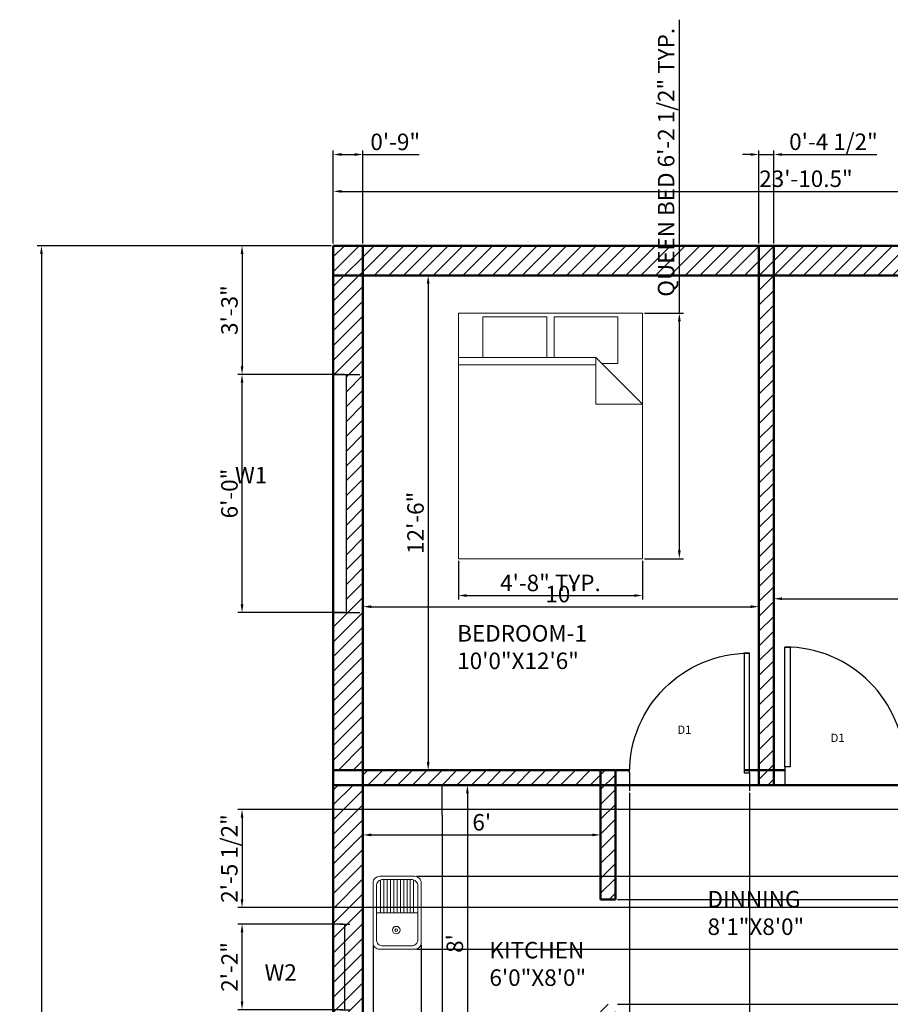
# Model space of a CAD drawing. Units: millimetres. Extents: x 2600 to 3013, y 1440 to 2066.
# Tile 3 of 4: x 2600 to 2864, y 1768 to 2066. Entities that reach past the tile are written whole.
import ezdxf

# ---------------------------------------------------------------- set-up
doc = ezdxf.new("R2010")
doc.units = ezdxf.units.MM
for name, color, linetype, lineweight in [('A-AREA-IDEN', 130, 'Continuous', 25), ('A-FLOR-CASE', 8, 'Continuous', 25), ('A-FLOR-FIXT', 160, 'Continuous', 18), ('A-WALL-PATT', 90, 'Continuous', 13), ('dimensions', 50, 'Continuous', 18), ('doors', 200, 'Continuous', 25), ('furniture', 160, 'Continuous', 18), ('text', 130, 'Continuous', 18), ('walls', 90, 'Continuous', 50), ('windows', 30, 'Continuous', 25)]:
    doc.layers.add(name, color=color, linetype=linetype, lineweight=lineweight)
doc.styles.get("Standard").update_dxf_attribs({"font": 'arial.ttf'})
doc.dimstyles.new('ISO-25', dxfattribs={"dimtxt": 5, "dimasz": 2.5, "dimexe": 1.25, "dimexo": 0.625, "dimtad": 1, "dimdec": 1, "dimlunit": 3, "dimtxsty": 'Standard', "dimcen": 2.5, "dimadec": 0, "dimazin": 0, "dimtfac": 1, "dimtdec": 1, "dimtmove": 0, "dimatfit": 3, "dimfxl": 1, "dimarcsym": 0})

# ---------------------------------------------------------------- blocks, each defined once
blk = doc.blocks.new('*U2')
for p, q in [((0, 0), (0, -6)), ((40, 0), (40, -6))]:
    blk.add_line(p, q)
blk.add_lwpolyline([(0, 0), (0, 40), (1.75, 40), (1.75, 0)], close=True)
blk.add_arc((0, 0), 40, 0, 90)
blk = doc.blocks.new('*U4')
for p, q in [((0, 4), (0, 0)), ((0, 2), (36, 2)), ((36, 4), (36, 0))]:
    blk.add_line(p, q)
blk = doc.blocks.new('*U6')
for p, q in [((0, 4), (0, 0)), ((36, 4), (36, 0)), ((0, 2), (36, 2))]:
    blk.add_line(p, q)
blk = doc.blocks.new('Bed - Queen')
for p, q in [((0, -80.00003), (0, 0)), ((0, 0), (59.99999, 0)), ((59.99999, 0), (59.99999, -80.00003)), ((7.99999, -1.2), (28.79998, -1.2)), ((7.99999, -14.4), (7.99999, -1.2)), ((28.79998, -1.2), (28.79998, -14.4)), ((31.19999, -1.2), (51.99999, -1.2)), ((31.19999, -14.4), (31.19999, -1.2)), ((51.99999, -1.2), (51.99999, -16.4)), ((0, -14.4), (44.8, -14.4)), ((59.99999, -29.6), (44.8, -14.4)), ((44.8, -14.4), (44.8, -29.6)), ((44.8, -16.8), (0, -16.8)), ((51.99999, -16.4), (46.79936, -16.4)), ((44.8, -29.6), (59.99999, -29.6)), ((59.99999, -80.00003), (0, -80.00003))]:
    blk.add_line(p, q)
blk = doc.blocks.new('*D10')
at = {"layer": 'Defpoints', "color": 0, "transparency": 16777216}
for p in [(2703.76, 1895.81), (2823.76, 1895.81), (2823.76, 1888.27)]:
    blk.add_point(p, dxfattribs=at)
at = {"layer": 'dimensions', "color": 0, "lineweight": -2, "transparency": 16777216}
for p, q in [((2703.76, 1895.19), (2703.76, 1887.02)), ((2823.76, 1895.19), (2823.76, 1887.02)), ((2706.26, 1888.27), (2821.26, 1888.27))]:
    blk.add_line(p, q, dxfattribs=at)
at = {"layer": 'dimensions', "color": 0, "transparency": 16777216}
for points in [[(2706.26, 1888.69), (2706.26, 1887.86), (2703.76, 1888.27)], [(2821.26, 1888.69), (2821.26, 1887.86), (2823.76, 1888.27)]]:
    blk.add_solid(points, dxfattribs=at)
at = {"layer": 'dimensions', "color": 0, "transparency": 16777216, "insert": (2763.76, 1891.45), "char_height": 5, "attachment_point": 5}
blk.add_mtext("10'", dxfattribs=at)
blk = doc.blocks.new('*D11')
at = {"layer": 'Defpoints', "color": 0, "transparency": 16777216}
for p in [(2714.32, 1988.68), (2714.32, 1838.68), (2723.51, 1838.68)]:
    blk.add_point(p, dxfattribs=at)
at = {"layer": 'dimensions', "color": 0, "lineweight": -2, "transparency": 16777216}
for p, q in [((2714.95, 1988.68), (2724.76, 1988.68)), ((2723.51, 1986.18), (2723.51, 1841.18)), ((2714.95, 1838.68), (2724.76, 1838.68))]:
    blk.add_line(p, q, dxfattribs=at)
at = {"layer": 'dimensions', "color": 0, "transparency": 16777216}
for points in [[(2723.1, 1986.18), (2723.93, 1986.18), (2723.51, 1988.68)], [(2723.1, 1841.18), (2723.93, 1841.18), (2723.51, 1838.68)]]:
    blk.add_solid(points, dxfattribs=at)
at = {"layer": 'dimensions', "color": 0, "transparency": 16777216, "insert": (2720.34, 1913.68), "char_height": 5, "attachment_point": 5, "rotation": 90}
blk.add_mtext('12\'-6"', dxfattribs=at)
blk = doc.blocks.new('*D12')
at = {"layer": 'Defpoints', "color": 0, "transparency": 16777216}
for p in [(2828.26, 1889.98), (2972.26, 1890.68), (2972.26, 1890.68)]:
    blk.add_point(p, dxfattribs=at)
at = {"layer": 'dimensions', "color": 0, "lineweight": -2, "transparency": 16777216}
for p, q in [((2828.26, 1890.6), (2828.26, 1891.93)), ((2830.76, 1890.68), (2969.76, 1890.68)), ((2972.26, 1891.3), (2972.26, 1891.93))]:
    blk.add_line(p, q, dxfattribs=at)
at = {"layer": 'dimensions', "color": 0, "transparency": 16777216}
for points in [[(2830.76, 1891.1), (2830.76, 1890.26), (2828.26, 1890.68)], [(2969.76, 1891.1), (2969.76, 1890.26), (2972.26, 1890.68)]]:
    blk.add_solid(points, dxfattribs=at)
at = {"layer": 'dimensions', "color": 0, "transparency": 16777216, "insert": (2900.26, 1893.81), "char_height": 5, "attachment_point": 5}
blk.add_mtext("12'", dxfattribs=at)
blk = doc.blocks.new('*D14')
at = {"layer": 'Defpoints', "color": 0, "transparency": 16777216}
for p in [(2735.41, 1834.18), (2735.41, 1738.18), (2735.41, 1738.18)]:
    blk.add_point(p, dxfattribs=at)
at = {"layer": 'dimensions', "color": 0, "lineweight": -2, "transparency": 16777216}
for p, q in [((2736.04, 1834.18), (2736.66, 1834.18)), ((2735.41, 1831.68), (2735.41, 1740.68)), ((2736.04, 1738.18), (2736.66, 1738.18))]:
    blk.add_line(p, q, dxfattribs=at)
at = {"layer": 'dimensions', "color": 0, "transparency": 16777216}
for points in [[(2735, 1831.68), (2735.83, 1831.68), (2735.41, 1834.18)], [(2735, 1740.68), (2735.83, 1740.68), (2735.41, 1738.18)]]:
    blk.add_solid(points, dxfattribs=at)
at = {"layer": 'dimensions', "color": 0, "transparency": 16777216, "insert": (2732.24, 1786.18), "char_height": 5, "attachment_point": 5, "rotation": 90}
blk.add_mtext("8'", dxfattribs=at)
blk = doc.blocks.new('*D15')
at = {"layer": 'Defpoints', "color": 0, "transparency": 16777216}
for p in [(2703.76, 1826.2), (2775.76, 1826.2), (2775.76, 1819.09)]:
    blk.add_point(p, dxfattribs=at)
at = {"layer": 'dimensions', "color": 0, "lineweight": -2, "transparency": 16777216}
for p, q in [((2703.76, 1825.58), (2703.76, 1817.84)), ((2775.76, 1825.58), (2775.76, 1817.84)), ((2706.26, 1819.09), (2773.26, 1819.09))]:
    blk.add_line(p, q, dxfattribs=at)
at = {"layer": 'dimensions', "color": 0, "transparency": 16777216}
for points in [[(2706.26, 1819.51), (2706.26, 1818.67), (2703.76, 1819.09)], [(2773.26, 1819.51), (2773.26, 1818.67), (2775.76, 1819.09)]]:
    blk.add_solid(points, dxfattribs=at)
at = {"layer": 'dimensions', "color": 0, "transparency": 16777216, "insert": (2739.76, 1822.27), "char_height": 5, "attachment_point": 5}
blk.add_mtext("6'", dxfattribs=at)
blk = doc.blocks.new('*D27')
at = {"layer": 'Defpoints', "color": 0, "transparency": 16777216}
for p in [(2981.26, 2014.15), (2694.76, 1997.68), (2981.26, 1997.68)]:
    blk.add_point(p, dxfattribs=at)
at = {"layer": 'dimensions', "color": 0, "lineweight": -2, "transparency": 16777216}
for p, q in [((2694.76, 1998.3), (2694.76, 2015.4)), ((2981.26, 1998.3), (2981.26, 2015.4)), ((2697.26, 2014.15), (2978.76, 2014.15))]:
    blk.add_line(p, q, dxfattribs=at)
at = {"layer": 'dimensions', "color": 0, "transparency": 16777216}
for points in [[(2697.26, 2014.57), (2697.26, 2013.74), (2694.76, 2014.15)], [(2978.76, 2014.57), (2978.76, 2013.74), (2981.26, 2014.15)]]:
    blk.add_solid(points, dxfattribs=at)
at = {"layer": 'dimensions', "color": 0, "transparency": 16777216, "insert": (2838.01, 2017.33), "char_height": 5, "attachment_point": 5}
blk.add_mtext('23\'-10.5"', dxfattribs=at)
blk = doc.blocks.new('*D28')
at = {"layer": 'Defpoints', "color": 0, "transparency": 16777216}
for p in [(2694.76, 1997.68), (2606.3, 1506.18), (2694.76, 1506.18)]:
    blk.add_point(p, dxfattribs=at)
at = {"layer": 'dimensions', "color": 0, "lineweight": -2, "transparency": 16777216}
for p, q in [((2694.13, 1997.68), (2605.05, 1997.68)), ((2606.3, 1995.18), (2606.3, 1508.68)), ((2694.13, 1506.18), (2605.05, 1506.18))]:
    blk.add_line(p, q, dxfattribs=at)
at = {"layer": 'dimensions', "color": 0, "transparency": 16777216}
for points in [[(2605.88, 1995.18), (2606.72, 1995.18), (2606.3, 1997.68)], [(2605.88, 1508.68), (2606.72, 1508.68), (2606.3, 1506.18)]]:
    blk.add_solid(points, dxfattribs=at)
at = {"layer": 'dimensions', "color": 0, "transparency": 16777216, "insert": (2603.12, 1751.93), "char_height": 5, "attachment_point": 5, "rotation": 90}
blk.add_mtext('40\'-11.5"', dxfattribs=at)
blk = doc.blocks.new('*D29')
at = {"layer": 'Defpoints', "color": 0, "transparency": 16777216}
for p in [(2788.48, 1977.23), (2799.64, 1977.23), (2788.48, 1902.81)]:
    blk.add_point(p, dxfattribs=at)
at = {"layer": 'dimensions', "color": 0, "lineweight": -2, "transparency": 16777216}
for p, q in [((2799.64, 1977.23), (2799.64, 2066.19)), ((2789.1, 1977.23), (2800.89, 1977.23)), ((2799.64, 1905.31), (2799.64, 1974.73)), ((2789.1, 1902.81), (2800.89, 1902.81))]:
    blk.add_line(p, q, dxfattribs=at)
at = {"layer": 'dimensions', "color": 0, "transparency": 16777216}
for points in [[(2799.22, 1974.73), (2800.06, 1974.73), (2799.64, 1977.23)], [(2799.22, 1905.31), (2800.06, 1905.31), (2799.64, 1902.81)]]:
    blk.add_solid(points, dxfattribs=at)
at = {"layer": 'dimensions', "color": 0, "transparency": 16777216, "insert": (2796.28, 2022.96), "char_height": 5, "attachment_point": 5, "rotation": 90}
blk.add_mtext('QUEEN BED 6\'-2 1/2" TYP.', dxfattribs=at)
blk = doc.blocks.new('*D30')
at = {"layer": 'Defpoints', "color": 0, "transparency": 16777216}
for p in [(2732.66, 1902.81), (2788.48, 1902.81), (2788.48, 1891.65)]:
    blk.add_point(p, dxfattribs=at)
at = {"layer": 'dimensions', "color": 0, "lineweight": -2, "transparency": 16777216}
for p, q in [((2732.66, 1902.19), (2732.66, 1890.4)), ((2788.48, 1902.19), (2788.48, 1890.4)), ((2735.16, 1891.65), (2785.98, 1891.65))]:
    blk.add_line(p, q, dxfattribs=at)
at = {"layer": 'dimensions', "color": 0, "transparency": 16777216}
for points in [[(2735.16, 1892.07), (2735.16, 1891.23), (2732.66, 1891.65)], [(2785.98, 1892.07), (2785.98, 1891.23), (2788.48, 1891.65)]]:
    blk.add_solid(points, dxfattribs=at)
at = {"layer": 'dimensions', "color": 0, "transparency": 16777216, "insert": (2760.57, 1894.83), "char_height": 5, "attachment_point": 5}
blk.add_mtext('4\'-8" TYP.', dxfattribs=at)
blk = doc.blocks.new('*D38')
at = {"layer": 'Defpoints', "color": 0, "transparency": 16777216}
for p in [(2703.76, 2025.33), (2694.76, 1997.68), (2703.76, 1997.68)]:
    blk.add_point(p, dxfattribs=at)
at = {"layer": 'dimensions', "color": 0, "lineweight": -2, "transparency": 16777216}
for p, q in [((2694.76, 1998.3), (2694.76, 2026.58)), ((2703.76, 1998.3), (2703.76, 2026.58)), ((2697.26, 2025.33), (2701.26, 2025.33)), ((2703.76, 2025.33), (2720.8, 2025.33))]:
    blk.add_line(p, q, dxfattribs=at)
at = {"layer": 'dimensions', "color": 0, "transparency": 16777216}
for points in [[(2697.26, 2025.75), (2697.26, 2024.91), (2694.76, 2025.33)], [(2701.26, 2025.75), (2701.26, 2024.91), (2703.76, 2025.33)]]:
    blk.add_solid(points, dxfattribs=at)
at = {"layer": 'dimensions', "color": 0, "transparency": 16777216, "insert": (2713.53, 2028.51), "char_height": 5, "attachment_point": 5}
blk.add_mtext('0\'-9"', dxfattribs=at)
blk = doc.blocks.new('*D39')
at = {"layer": 'Defpoints', "color": 0, "transparency": 16777216}
for p in [(2828.26, 2025.33), (2823.76, 1997.68), (2828.26, 1997.68)]:
    blk.add_point(p, dxfattribs=at)
at = {"layer": 'dimensions', "color": 0, "lineweight": -2, "transparency": 16777216}
for p, q in [((2823.76, 1998.3), (2823.76, 2026.58)), ((2828.26, 1998.3), (2828.26, 2026.58)), ((2821.26, 2025.33), (2818.76, 2025.33)), ((2823.76, 2025.33), (2828.26, 2025.33)), ((2830.76, 2025.33), (2859.45, 2025.33))]:
    blk.add_line(p, q, dxfattribs=at)
at = {"layer": 'dimensions', "color": 0, "transparency": 16777216}
for points in [[(2821.26, 2025.75), (2821.26, 2024.91), (2823.76, 2025.33)], [(2830.76, 2025.75), (2830.76, 2024.91), (2828.26, 2025.33)]]:
    blk.add_solid(points, dxfattribs=at)
at = {"layer": 'dimensions', "color": 0, "transparency": 16777216, "insert": (2846.35, 2028.54), "char_height": 5, "attachment_point": 5}
blk.add_mtext('0\'-4 1/2"', dxfattribs=at)
blk = doc.blocks.new('*D40')
at = {"layer": 'Defpoints', "color": 0, "transparency": 16777216}
for p in [(2667.11, 1958.65), (2698.77, 1958.65), (2698.77, 1886.48)]:
    blk.add_point(p, dxfattribs=at)
at = {"layer": 'dimensions', "color": 0, "lineweight": -2, "transparency": 16777216}
for p, q in [((2698.14, 1958.65), (2665.86, 1958.65)), ((2667.11, 1888.98), (2667.11, 1956.15)), ((2698.14, 1886.48), (2665.86, 1886.48))]:
    blk.add_line(p, q, dxfattribs=at)
at = {"layer": 'dimensions', "color": 0, "transparency": 16777216}
for points in [[(2666.69, 1956.15), (2667.52, 1956.15), (2667.11, 1958.65)], [(2666.69, 1888.98), (2667.52, 1888.98), (2667.11, 1886.48)]]:
    blk.add_solid(points, dxfattribs=at)
at = {"layer": 'dimensions', "color": 0, "transparency": 16777216, "insert": (2663.93, 1922.56), "char_height": 5, "attachment_point": 5, "rotation": 90}
blk.add_mtext('6\'-0"', dxfattribs=at)
blk = doc.blocks.new('*D41')
at = {"layer": 'Defpoints', "color": 0, "transparency": 16777216}
for p in [(2667.11, 1792.07), (2698.28, 1792.07), (2698.28, 1766.09)]:
    blk.add_point(p, dxfattribs=at)
at = {"layer": 'dimensions', "color": 0, "lineweight": -2, "transparency": 16777216}
for p, q in [((2697.66, 1792.07), (2665.86, 1792.07)), ((2667.11, 1768.59), (2667.11, 1789.57)), ((2697.66, 1766.09), (2665.86, 1766.09))]:
    blk.add_line(p, q, dxfattribs=at)
at = {"layer": 'dimensions', "color": 0, "transparency": 16777216}
for points in [[(2666.69, 1789.57), (2667.52, 1789.57), (2667.11, 1792.07)], [(2666.69, 1768.59), (2667.52, 1768.59), (2667.11, 1766.09)]]:
    blk.add_solid(points, dxfattribs=at)
at = {"layer": 'dimensions', "color": 0, "transparency": 16777216, "insert": (2663.97, 1779.08), "char_height": 5, "attachment_point": 5, "rotation": 90}
blk.add_mtext('2\'-2"', dxfattribs=at)
blk = doc.blocks.new('*D43')
at = {"layer": 'Defpoints', "color": 0, "transparency": 16777216}
for p in [(2784.55, 1832.44), (2820.86, 1832.44), (2820.86, 1444.53)]:
    blk.add_point(p, dxfattribs=at)
at = {"layer": 'dimensions', "color": 0, "lineweight": -2, "transparency": 16777216}
for p, q in [((2784.55, 1831.81), (2784.55, 1443.28)), ((2820.86, 1831.81), (2820.86, 1443.28)), ((2787.05, 1444.53), (2818.36, 1444.53))]:
    blk.add_line(p, q, dxfattribs=at)
at = {"layer": 'dimensions', "color": 0, "transparency": 16777216}
for points in [[(2787.05, 1444.94), (2787.05, 1444.11), (2784.55, 1444.53)], [(2818.36, 1444.94), (2818.36, 1444.11), (2820.86, 1444.53)]]:
    blk.add_solid(points, dxfattribs=at)
at = {"layer": 'dimensions', "color": 0, "transparency": 16777216, "insert": (2802.7, 1447.74), "char_height": 5, "attachment_point": 5}
blk.add_mtext('3\'-0 1/2"', dxfattribs=at)
blk = doc.blocks.new('*D44')
at = {"layer": 'Defpoints', "color": 0, "transparency": 16777216}
for p in [(2883.26, 1826.8), (2667.11, 1797.08), (2883.26, 1797.08)]:
    blk.add_point(p, dxfattribs=at)
at = {"layer": 'dimensions', "color": 0, "lineweight": -2, "transparency": 16777216}
for p, q in [((2882.63, 1826.8), (2665.86, 1826.8)), ((2667.11, 1824.3), (2667.11, 1799.58)), ((2882.63, 1797.08), (2665.86, 1797.08))]:
    blk.add_line(p, q, dxfattribs=at)
at = {"layer": 'dimensions', "color": 0, "transparency": 16777216}
for points in [[(2666.69, 1824.3), (2667.52, 1824.3), (2667.11, 1826.8)], [(2666.69, 1799.58), (2667.52, 1799.58), (2667.11, 1797.08)]]:
    blk.add_solid(points, dxfattribs=at)
at = {"layer": 'dimensions', "color": 0, "transparency": 16777216, "insert": (2663.9, 1811.94), "char_height": 5, "attachment_point": 5, "rotation": 90}
blk.add_mtext('2\'-5 1/2"', dxfattribs=at)
blk = doc.blocks.new('*D47')
at = {"layer": 'Defpoints', "color": 0, "transparency": 16777216}
for p in [(2780.26, 1799.5), (3008.91, 1799.5), (2780.26, 1767.75)]:
    blk.add_point(p, dxfattribs=at)
at = {"layer": 'dimensions', "color": 0, "lineweight": -2, "transparency": 16777216}
for p, q in [((2780.88, 1799.5), (3010.16, 1799.5)), ((3008.91, 1770.25), (3008.91, 1797)), ((2780.88, 1767.75), (3010.16, 1767.75))]:
    blk.add_line(p, q, dxfattribs=at)
at = {"layer": 'dimensions', "color": 0, "transparency": 16777216}
for points in [[(3008.49, 1797), (3009.32, 1797), (3008.91, 1799.5)], [(3008.49, 1770.25), (3009.32, 1770.25), (3008.91, 1767.75)]]:
    blk.add_solid(points, dxfattribs=at)
at = {"layer": 'dimensions', "color": 0, "transparency": 16777216, "insert": (3005.73, 1783.63), "char_height": 5, "attachment_point": 5, "rotation": 90}
blk.add_mtext('2\'-8"', dxfattribs=at)
blk = doc.blocks.new('*D48')
at = {"layer": 'Defpoints', "color": 0, "transparency": 16777216}
for p in [(2706.82, 1786.43), (2721.39, 1786.43), (2721.39, 1444.53)]:
    blk.add_point(p, dxfattribs=at)
at = {"layer": 'dimensions', "color": 0, "lineweight": -2, "transparency": 16777216}
for p, q in [((2706.82, 1785.8), (2706.82, 1443.28)), ((2721.39, 1785.8), (2721.39, 1443.28)), ((2709.32, 1444.53), (2718.89, 1444.53)), ((2721.39, 1444.53), (2749.61, 1444.53))]:
    blk.add_line(p, q, dxfattribs=at)
at = {"layer": 'dimensions', "color": 0, "transparency": 16777216}
for points in [[(2709.32, 1444.94), (2709.32, 1444.11), (2706.82, 1444.53)], [(2718.89, 1444.94), (2718.89, 1444.11), (2721.39, 1444.53)]]:
    blk.add_solid(points, dxfattribs=at)
at = {"layer": 'dimensions', "color": 0, "transparency": 16777216, "insert": (2736.75, 1447.74), "char_height": 5, "attachment_point": 5}
blk.add_mtext('1\'-2 1/2"', dxfattribs=at)
blk = doc.blocks.new('*D49')
at = {"layer": 'Defpoints', "color": 0, "transparency": 16777216}
for p in [(2719.39, 1806.57), (3008.91, 1806.57), (2719.39, 1784.43)]:
    blk.add_point(p, dxfattribs=at)
at = {"layer": 'dimensions', "color": 0, "lineweight": -2, "transparency": 16777216}
for p, q in [((2720.01, 1806.57), (3010.16, 1806.57)), ((3008.91, 1786.93), (3008.91, 1804.07)), ((2720.01, 1784.43), (3010.16, 1784.43))]:
    blk.add_line(p, q, dxfattribs=at)
at = {"layer": 'dimensions', "color": 0, "transparency": 16777216}
for points in [[(3008.49, 1804.07), (3009.32, 1804.07), (3008.91, 1806.57)], [(3008.49, 1786.93), (3009.32, 1786.93), (3008.91, 1784.43)]]:
    blk.add_solid(points, dxfattribs=at)
at = {"layer": 'dimensions', "color": 0, "transparency": 16777216, "insert": (3005.73, 1795.5), "char_height": 5, "attachment_point": 5, "rotation": 90}
blk.add_mtext('1\'-10"', dxfattribs=at)
blk = doc.blocks.new('*D50')
at = {"layer": 'Defpoints', "color": 0, "transparency": 16777216}
for p in [(2694.76, 1997.68), (2667.11, 1958.65), (2698.77, 1958.65)]:
    blk.add_point(p, dxfattribs=at)
at = {"layer": 'dimensions', "color": 0, "lineweight": -2, "transparency": 16777216}
for p, q in [((2694.13, 1997.68), (2665.86, 1997.68)), ((2667.11, 1995.18), (2667.11, 1961.15)), ((2698.14, 1958.65), (2665.86, 1958.65))]:
    blk.add_line(p, q, dxfattribs=at)
at = {"layer": 'dimensions', "color": 0, "transparency": 16777216}
for points in [[(2666.69, 1995.18), (2667.52, 1995.18), (2667.11, 1997.68)], [(2666.69, 1961.15), (2667.52, 1961.15), (2667.11, 1958.65)]]:
    blk.add_solid(points, dxfattribs=at)
at = {"layer": 'dimensions', "color": 0, "transparency": 16777216, "insert": (2663.93, 1978.16), "char_height": 5, "attachment_point": 5, "rotation": 90}
blk.add_mtext('3\'-3"', dxfattribs=at)

msp = doc.modelspace()

# ---------------------------------------------------------------- hatches: boundary and pattern name
at = {"layer": 'A-WALL-PATT'}
h = msp.add_hatch(dxfattribs=at)
h.set_pattern_fill('ANSI31', color=256)
h.paths.add_polyline_path([(2972.26, 1997.68), (2828.26, 1997.68), (2828.26, 1988.68), (2972.26, 1988.68)])
h.paths.add_polyline_path([(2823.76, 1997.68), (2703.76, 1997.68), (2703.76, 1988.68), (2823.76, 1988.68)])
h.paths.add_polyline_path([(2828.26, 1997.68), (2823.76, 1997.68), (2823.76, 1988.68), (2828.26, 1988.68)])
h.paths.add_polyline_path([(2703.76, 1997.68), (2694.76, 1997.68), (2694.76, 1988.68), (2703.76, 1988.68)])
h.paths.add_polyline_path([(2703.76, 1988.68), (2694.76, 1988.68), (2694.76, 1958.65), (2698.77, 1958.65), (2698.77, 1886.48), (2694.76, 1886.48), (2694.76, 1838.68), (2703.76, 1838.68)])
h.paths.add_polyline_path([(2703.76, 1733.68), (2694.76, 1733.68), (2694.76, 1612.68), (2703.76, 1612.68)])
h.paths.add_polyline_path([(2703.76, 1608.18), (2694.76, 1608.18), (2694.76, 1506.18), (2703.76, 1506.18)])
h.paths.add_polyline_path([(2703.76, 1612.68), (2694.76, 1612.68), (2694.76, 1608.18), (2703.76, 1608.18)])
h.paths.add_polyline_path([(2823.76, 1612.68), (2703.76, 1612.68), (2703.76, 1608.18), (2823.76, 1608.18)])
h.paths.add_polyline_path([(2972.26, 1611.68), (2869.05, 1611.68, -0.005663), (2869.06, 1610.86), (2869.06, 1607.18), (2972.26, 1607.18)])
h.paths.add_polyline_path([(2981.26, 1607.18), (2972.26, 1607.18), (2972.26, 1506.18), (2981.26, 1506.18)])
h.paths.add_polyline_path([(2981.26, 1611.68), (2972.26, 1611.68), (2972.26, 1607.18), (2981.26, 1607.18)])
h.paths.add_polyline_path([(2828.26, 1569.75), (2824.68, 1569.8, -0.006355), (2823.76, 1569.82), (2823.76, 1506.18), (2828.26, 1506.18)])
h.paths.add_polyline_path([(2828.26, 1733.68), (2823.76, 1733.68), (2823.76, 1612.68), (2828.26, 1612.68)])
h.paths.add_polyline_path([(2981.26, 1783.68), (2972.26, 1783.68), (2972.26, 1611.68), (2981.26, 1611.68)])
h.paths.add_polyline_path([(2972.26, 1838.68), (2883.26, 1838.68), (2883.26, 1834.18), (2972.26, 1834.18)])
h.paths.add_polyline_path([(2981.26, 1838.68), (2972.26, 1838.68), (2972.26, 1834.18), (2981.26, 1834.18)])
h.paths.add_polyline_path([(2981.26, 1834.18), (2972.26, 1834.18), (2972.26, 1788.18), (2981.26, 1788.18)])
h.paths.add_polyline_path([(2981.26, 1988.68), (2972.26, 1988.68), (2972.26, 1952.13), (2976.27, 1952.13), (2976.27, 1879.95), (2972.26, 1879.95), (2972.26, 1838.68), (2981.26, 1838.68)])
h.paths.add_polyline_path([(2828.26, 1988.68), (2823.76, 1988.68), (2823.76, 1838.68), (2828.26, 1838.68)])
h.paths.add_polyline_path([(2780.26, 1834.18), (2775.76, 1834.18), (2775.76, 1799.5), (2780.26, 1799.5)])
h.paths.add_polyline_path([(2775.76, 1838.68), (2703.76, 1838.68), (2703.76, 1834.18), (2775.76, 1834.18)])
h.paths.add_polyline_path([(2780.26, 1838.68), (2775.76, 1838.68), (2775.76, 1834.18), (2780.26, 1834.18)])
h.paths.add_polyline_path([(2828.26, 1838.68), (2823.76, 1838.68), (2823.76, 1834.18), (2828.26, 1834.18)])
h.paths.add_polyline_path([(2883.26, 1838.68), (2878.76, 1838.68), (2878.76, 1834.18), (2883.26, 1834.18)])
h.paths.add_polyline_path([(2886.68, 1812.39), (2892.39, 1812.39), (2892.39, 1817.54), (2886.68, 1817.54)], flags=9)
h = msp.add_hatch(dxfattribs=at)
h.set_pattern_fill('ANSI31', color=256)
h.paths.add_polyline_path([(2703.76, 1834.18), (2694.76, 1834.18), (2694.76, 1738.18), (2703.76, 1738.18)])
h.paths.add_polyline_path([(2780.26, 1767.75), (2775.76, 1767.75), (2775.76, 1738.18), (2780.26, 1738.18)])
h.paths.add_polyline_path([(2972.26, 1506.18), (2868.8, 1506.18, -0.033203), (2869.12, 1501.37), (2869.12, 1497.18), (2972.26, 1497.18)])
h.paths.add_polyline_path([(2981.26, 1506.18), (2972.26, 1506.18), (2972.26, 1497.18), (2981.26, 1497.18)])
h.paths.add_polyline_path([(2823.76, 1506.18), (2703.76, 1506.18), (2703.76, 1497.18), (2823.76, 1497.18)])
h.paths.add_polyline_path([(2828.26, 1506.18), (2823.76, 1506.18), (2823.76, 1497.18), (2828.26, 1497.18)])
h.paths.add_polyline_path([(2832.8, 1506.18), (2828.26, 1506.18), (2828.26, 1497.18), (2832.8, 1497.18), (2832.8, 1501.37)])
h.paths.add_polyline_path([(2703.76, 1506.18), (2694.76, 1506.18), (2694.76, 1497.18), (2703.76, 1497.18)])
h.paths.add_polyline_path([(2981.26, 1997.68), (2972.26, 1997.68), (2972.26, 1988.68), (2981.26, 1988.68)])

# ---------------------------------------------------------------- linework, layer by layer
at = {"layer": 'A-FLOR-CASE'}
for q in [(2727.76, 1834.18), (2727.76, 1762.18)]:
    msp.add_line((2727.76, 1825.08), q, dxfattribs=at)
at = {"layer": 'A-FLOR-FIXT'}
for p, q in [((2710.11, 1795.5), (2710.11, 1805.57)), ((2711.11, 1795.5), (2711.11, 1805.57)), ((2712.11, 1795.5), (2712.11, 1805.57)), ((2713.11, 1795.5), (2713.11, 1805.57)), ((2714.11, 1795.5), (2714.11, 1805.57)), ((2715.11, 1795.5), (2715.11, 1805.57)), ((2716.11, 1795.5), (2716.11, 1805.57)), ((2717.11, 1795.5), (2717.11, 1805.57)), ((2718.11, 1795.5), (2718.11, 1805.57)), ((2709.11, 1795.5), (2709.11, 1805.44)), ((2719.11, 1795.5), (2719.11, 1805.44)), ((2707.82, 1795.5), (2720.39, 1795.5))]:
    msp.add_line(p, q, dxfattribs=at)
for points in [[(2708.82, 1806.57), (2719.39, 1806.57, -0.414214), (2721.39, 1804.57), (2721.39, 1786.43, -0.414214), (2719.39, 1784.43), (2708.82, 1784.43, -0.414214), (2706.82, 1786.43), (2706.82, 1804.57, -0.414214)], [(2709.82, 1805.57), (2718.39, 1805.57, -0.414214), (2720.39, 1803.57), (2720.39, 1787.43, -0.414214), (2718.39, 1785.43), (2709.82, 1785.43, -0.414214), (2707.82, 1787.43), (2707.82, 1803.57, -0.414214)]]:
    msp.add_lwpolyline(points, format="xyb", close=True, dxfattribs=at)
for radius in [1.14, 0.401]:
    msp.add_circle((2713.85, 1790.24), radius, dxfattribs=at)
at = {"layer": 'walls'}
for p, q in [((2694.76, 1997.68), (2694.76, 1497.18)), ((2694.76, 1997.68), (2981.26, 1997.68)), ((2703.76, 1997.68), (2703.76, 1497.18)), ((2823.76, 1997.68), (2823.76, 1834.18)), ((2823.76, 1997.68), (2823.76, 1834.18)), ((2823.76, 1997.68), (2823.76, 1834.18)), ((2828.26, 1997.68), (2828.26, 1834.18)), ((2828.26, 1997.68), (2828.26, 1834.18)), ((2828.26, 1997.68), (2828.26, 1834.18)), ((2694.76, 1988.68), (2981.26, 1988.68)), ((2694.76, 1838.68), (2784.55, 1838.68)), ((2694.76, 1838.68), (2784.55, 1838.68)), ((2775.76, 1838.68), (2775.76, 1799.5)), ((2775.76, 1838.68), (2775.76, 1799.5)), ((2780.26, 1838.68), (2780.26, 1799.5)), ((2780.26, 1838.68), (2780.26, 1799.5)), ((2819.27, 1838.68), (2828.26, 1838.68)), ((2819.27, 1838.68), (2831.64, 1838.68)), ((2694.76, 1834.18), (2828.26, 1834.18)), ((2694.76, 1834.18), (2981.26, 1834.18)), ((2775.76, 1799.5), (2780.26, 1799.5))]:
    msp.add_line(p, q, dxfattribs=at)

# ---------------------------------------------------------------- block references
at = {"layer": 'doors', "yscale": 0.9079361683412358, "zscale": 0.9079361683412358}
for p, xscale in [((2820.86, 1837.88), -0.9079361683412358), ((2831.64, 1839.73), 0.9079361683412358)]:
    msp.add_blockref('*U2', p, dxfattribs=dict(at, xscale=xscale))
at = {"layer": 'furniture', "xscale": 0.9302566542625909, "yscale": 0.9302566542625909, "zscale": 0.9302566542625909}
msp.add_blockref('Bed - Queen', (2732.66, 1977.23), dxfattribs=at)
at = {"layer": 'windows', "rotation": 90}
for name, p, xscale, yscale, zscale in [('*U6', (2702.78, 1886.48), 2.004851231759801, 2.004851231759801, 2.004851231759801), ('*U4', (2699.73, 1766.09), 0.7216899638288952, 0.7216899638288952, 0.7216899638288952)]:
    msp.add_blockref(name, p, dxfattribs=dict(at, xscale=xscale, yscale=yscale, zscale=zscale))

# ---------------------------------------------------------------- texts
at = {"layer": 'A-AREA-IDEN', "char_height": 5, "attachment_point": 1}
for s, width, insert in [('BEDROOM-1\\P10\'0"X12\'6"', 36.9462, (2732.31, 1882.69)), ('DINNING\\P8\'1"X8\'0"', 53.5963, (2808.18, 1802.11)), ('KITCHEN\\P6\'0"X8\'0"', 20.7668, (2742.08, 1786.67))]:
    msp.add_mtext_dynamic_manual_height_columns(s, width=width, gutter_width=12.5, heights=[0], dxfattribs=dict(at, insert=insert))
at = {"layer": 'text', "attachment_point": 1}
for s, width, insert, char_height in [('W1', 8.5835, (2664.98, 1930.62), 5), ('D1', 8.1744, (2799.06, 1852.22), 2.5), ('D1', 7.2576, (2845.5, 1849.77), 2.5), ('W2', 10.7214, (2673.93, 1779.88), 5)]:
    msp.add_mtext_dynamic_manual_height_columns(s, width=width, gutter_width=12.5, heights=[0], dxfattribs=dict(at, insert=insert, char_height=char_height))

# ---------------------------------------------------------------- dimensions: what is measured, and where the dimension line sits
at = {"layer": 'dimensions'}
dim = msp.add_linear_dim(base=(2799.64, 1977.23), p1=(2788.48, 1902.81), p2=(2788.48, 1977.23), angle=90, text='QUEEN BED <> TYP.', dimstyle='ISO-25', override={"dimdec": 1, "dimlfac": 1, "dimrnd": 0, "dimzin": 1, "dimdsep": 46, "dimlunit": 4, "dimfrac": 2}, dxfattribs=at)
dim.commit()
dim.dimension.update_dxf_attribs({"geometry": '*D29', "text_midpoint": (2796.28, 2022.96)})
for base, p1, p2, override, picture, middle in [((2828.26, 2025.33), (2823.76, 1997.68), (2828.26, 1997.68), {"dimdec": 1, "dimlfac": 1, "dimrnd": 0, "dimzin": 1, "dimdsep": 46, "dimlunit": 4, "dimfrac": 2}, '*D39', (2846.35, 2028.54)), ((2703.76, 2025.33), (2694.76, 1997.68), (2703.76, 1997.68), {"dimdec": 1, "dimlfac": 1, "dimrnd": 0, "dimzin": 1, "dimdsep": 46, "dimlunit": 4, "dimfrac": 2}, '*D38', (2713.53, 2028.51)), ((2981.26, 2014.15), (2694.76, 1997.68), (2981.26, 1997.68), {"dimclrd": 0, "dimclre": 0, "dimclrt": 0}, '*D27', (2838.01, 2017.33)), ((2823.76, 1888.27), (2703.76, 1895.81), (2823.76, 1895.81), {"dimclrd": 0, "dimclre": 0, "dimclrt": 0}, '*D10', (2763.76, 1891.45)), ((2972.26, 1890.68), (2828.26, 1889.98), (2972.26, 1890.68), {"dimclrd": 0, "dimclre": 0, "dimclrt": 0}, '*D12', (2900.26, 1893.81)), ((2820.86, 1444.53), (2784.55, 1832.44), (2820.86, 1832.44), {"dimdec": 1, "dimlfac": 1, "dimrnd": 0, "dimzin": 1, "dimdsep": 46, "dimlunit": 4, "dimfrac": 2}, '*D43', (2802.7, 1447.74)), ((2775.76, 1819.09), (2703.76, 1826.2), (2775.76, 1826.2), {"dimclrd": 0, "dimclre": 0, "dimclrt": 0}, '*D15', (2739.76, 1822.27)), ((2721.39, 1444.53), (2706.82, 1786.43), (2721.39, 1786.43), {"dimdec": 1, "dimlfac": 1, "dimrnd": 0, "dimzin": 1, "dimdsep": 46, "dimlunit": 4, "dimfrac": 2}, '*D48', (2736.75, 1447.74))]:
    dim = msp.add_linear_dim(base=base, p1=p1, p2=p2, dimstyle='ISO-25', override=override, dxfattribs=at)
    dim.commit()
    dim.dimension.update_dxf_attribs({"geometry": picture, "text_midpoint": middle})
for base, p1, p2, override, picture, middle in [((2606.3, 1506.18), (2694.76, 1997.68), (2694.76, 1506.18), {"dimclrd": 0, "dimclre": 0, "dimclrt": 0}, '*D28', (2603.12, 1751.93)), ((2667.11, 1958.65), (2694.76, 1997.68), (2698.77, 1958.65), {"dimdec": 1, "dimlfac": 1, "dimrnd": 0, "dimzin": 1, "dimdsep": 46, "dimlunit": 4, "dimfrac": 2}, '*D50', (2663.93, 1978.16)), ((2723.51, 1838.68), (2714.32, 1988.68), (2714.32, 1838.68), {"dimclrd": 0, "dimclre": 0, "dimclrt": 0}, '*D11', (2720.34, 1913.68)), ((2667.11, 1958.65), (2698.77, 1886.48), (2698.77, 1958.65), {"dimdec": 1, "dimlfac": 1, "dimrnd": 0, "dimzin": 1, "dimdsep": 46, "dimlunit": 4, "dimfrac": 2}, '*D40', (2663.93, 1922.56)), ((2735.41, 1738.18), (2735.41, 1834.18), (2735.41, 1738.18), {"dimclrd": 0, "dimclre": 0, "dimclrt": 0}, '*D14', (2732.24, 1786.18)), ((2667.11, 1797.08), (2883.26, 1826.8), (2883.26, 1797.08), {"dimdec": 1, "dimlfac": 1, "dimrnd": 0, "dimzin": 1, "dimdsep": 46, "dimlunit": 4, "dimfrac": 2}, '*D44', (2663.9, 1811.94)), ((3008.91, 1806.57), (2719.39, 1784.43), (2719.39, 1806.57), {"dimdec": 1, "dimlfac": 1, "dimrnd": 0, "dimzin": 1, "dimdsep": 46, "dimlunit": 4, "dimfrac": 2}, '*D49', (3005.73, 1795.5)), ((3008.9057, 1799.5016), (2780.2557, 1767.7507), (2780.2557, 1799.5016), {"dimdec": 1, "dimlfac": 1, "dimrnd": 0, "dimzin": 1, "dimdsep": 46, "dimlunit": 4, "dimfrac": 2}, '*D47', (3005.7279, 1783.6262)), ((2667.11, 1792.07), (2698.28, 1766.09), (2698.28, 1792.07), {"dimdec": 1, "dimlfac": 1, "dimrnd": 0, "dimzin": 1, "dimdsep": 46, "dimlunit": 4, "dimfrac": 2}, '*D41', (2663.97, 1779.08))]:
    dim = msp.add_linear_dim(base=base, p1=p1, p2=p2, angle=90, dimstyle='ISO-25', override=override, dxfattribs=at)
    dim.commit()
    dim.dimension.update_dxf_attribs({"geometry": picture, "text_midpoint": middle})
dim = msp.add_linear_dim(base=(2788.48, 1891.65), p1=(2732.66, 1902.81), p2=(2788.48, 1902.81), text='<> TYP.', dimstyle='ISO-25', override={"dimdec": 1, "dimlfac": 1, "dimrnd": 0, "dimzin": 1, "dimdsep": 46, "dimlunit": 4, "dimfrac": 2}, dxfattribs=at)
dim.commit()
dim.dimension.update_dxf_attribs({"geometry": '*D30', "text_midpoint": (2760.57, 1894.83)})

doc.saveas('drawing.dxf')
